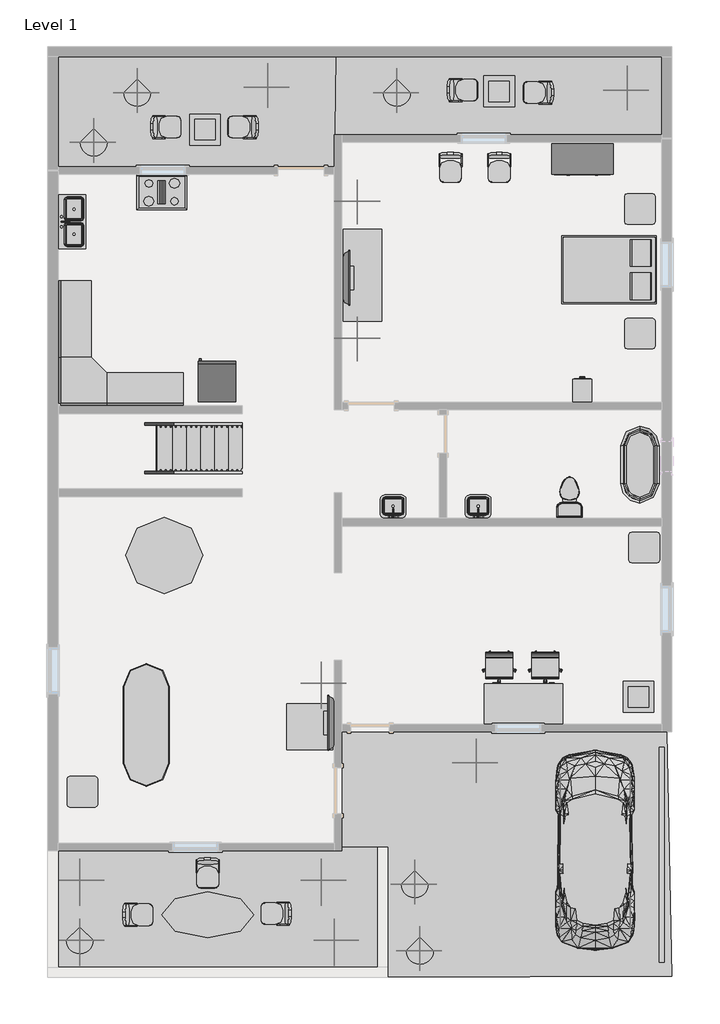
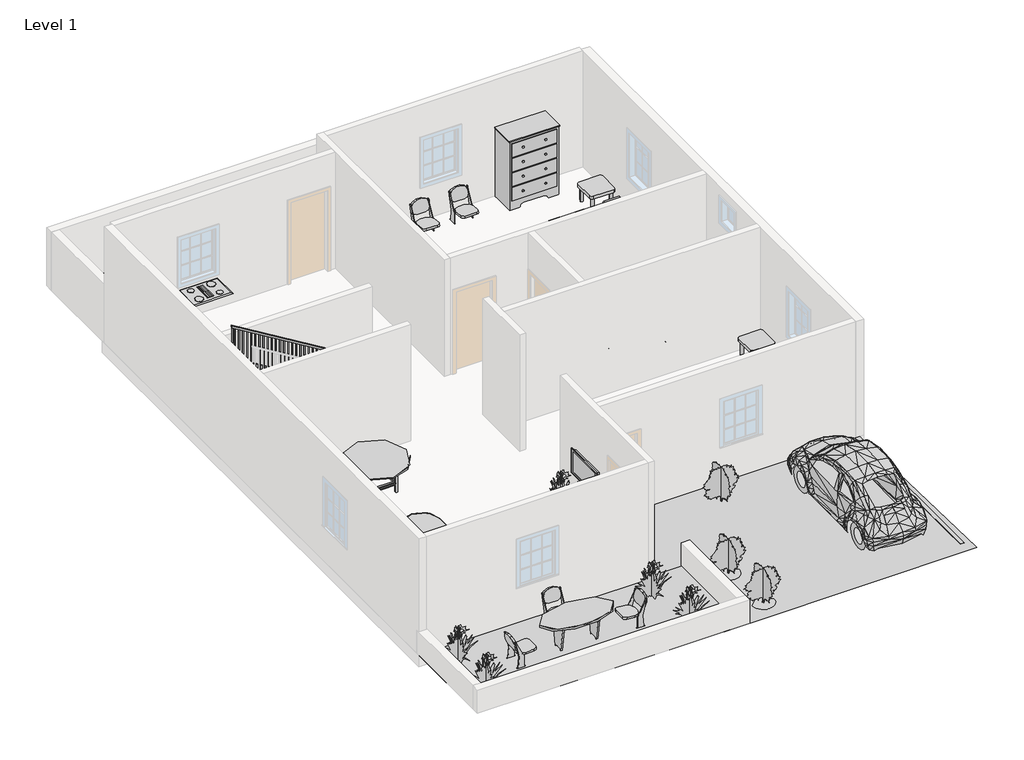
# One storey, part 2 of 2: 30 furniture elements, 15 geographic elements, 8 proxies, 6 flow terminals, 2 members, 1 railing, 1 stair flight.
"""IFC4 building model written with IfcOpenShell, lengths in millimetres."""

from ifc_helpers import new_model, si_unit, frame, origin, place, context, project, spatial, polyline, outline, extrude, triangles, transform, mapped, element, save
from components import proxy_bb1e6e30, parking_space_9_x_18_90_deg_fdd9e8f5, rpc_beetle_rpc_beetle_3ce7ba48, proxy_a13a33b2, flow_terminal_2b63360b, flow_terminal_a53be723, flow_terminal_62a433f7, toilet_domestic_3d_toilet_domestic_3d_f7549cf7, toilet_domestic_3d_toilet_domestic_3d_183bbd19, flow_terminal_b374fae2, furniture_1070mm_7a3aaa4f, furniture_c8abb964, furniture_552c1472, chair_task_chair_task_b7f3823b, furniture_013ab306, furniture_9fa109b2, m_table_rectangular_0915_x_0915mm_8578315f, furniture_3d1d9cbc, furniture_b5c51a22, furniture_e05f6f82, furniture_bbcc68ce, furniture_027a2ad9, furniture_5d68651d, furniture_a5b052b6, furniture_45e3acac, rpc_plant_tropical_55f6ff97, rpc_plant_tropical_agave_1_5_93a2a214, rpc_plant_tropical_jungle_flame_3_9c4808c2, stair_flight_159ea243

model = new_model("IFC4")

# Units and contexts
model_context = context("Model", 3, world=origin())
ifc_project = project(units=[si_unit("LENGTHUNIT", "METRE", prefix="MILLI")], contexts=[model_context])

# Site, building, storey
site = spatial("IfcSite", under=ifc_project)
building = spatial("IfcBuilding", under=site)
storey = spatial("IfcBuildingStorey", under=building, Name="Level 1", Elevation=0.0)

# Proxies
placement = place(None, origin())
element("IfcBuildingElementProxy", 1, Name="Building Element Proxy", at=placement, inside=storey, context=model_context, shape_type="Tessellation", body=[
    triangles([(-6254.9251831, -3080.6256248, 0.0), (-6254.9251831, -5671.4259155, 0.0), (501.4745868, -5671.4259155, 0.0), (501.4745868, -3080.6256248, 0.0), (-412.9254132, -3156.8256248, 0.0)], [[1, 2, 5], [5, 3, 4], [3, 5, 2], [5, 4, 1]], closed=False),
])
element("IfcBuildingElementProxy", 2, Name="Building Element Proxy", at=placement, inside=storey, context=model_context, shape_type="Tessellation", body=[
    triangles([(-412.9254132, -794.6256975, 0.0), (-412.9254132, -3156.8256248, 0.0), (6040.245845, -794.6256975, 0.0), (6140.2746231, -5646.0257217, 0.0), (501.4745868, -5671.4259155, 0.0), (-235.1254193, -693.0257217, 0.0), (526.8745989, -693.0257217, 0.0), (-514.5254253, -1505.8256733, 0.0), (-514.5254253, -2420.2256733, 0.0)], [[7, 8, 9], [6, 1, 8], [9, 2, 7], [5, 4, 3], [7, 6, 8], [2, 3, 7], [2, 5, 3]], closed=False),
])
element("IfcBuildingElementProxy", 3, Name="Building Element Proxy", at=placement, inside=storey, context=model_context, shape_type="Tessellation", body=[
    triangles([(-6051.7253769, 12616.5740845, 0.0), (-6051.7253769, 10432.1736969, 0.0), (-565.3254132, 10432.1736969, 0.0), (-533.6047113, 12616.5740845, 0.0)], [[1, 2, 3], [3, 4, 1]], closed=False),
])
element("IfcBuildingElementProxy", 4, Name="Building Element Proxy", at=placement, inside=storey, context=model_context, shape_type="Tessellation", body=[
    triangles([(-565.3254132, 11067.174472, 0.0), (-561.2836905, 12616.5740845, 0.0), (5937.0748169, 11067.174472, 0.0), (5937.0748169, 12616.5740845, 0.0)], [[2, 1, 3], [3, 4, 2]], closed=False),
])
proxy_shape = proxy_bb1e6e30(model_context)
element("IfcBuildingElementProxy", 5, Name="Cook Top-4 Unit : 36\" x 20\"", ObjectType="Cook Top-4 Unit : 36\" x 20\"", at=placement, inside=storey, context=model_context, shape_type="MappedRepresentation", body=[
    mapped(proxy_shape, transform((-3994.3254147, 9924.1742707, 0.0), x_axis=(1.0, 0.0, 0.0), y_axis=(0.0, 1.0, 0.0), z_axis=(0.0, 0.0, 1.0))),
])
parking_space_9_x_18_90_deg_shape = parking_space_9_x_18_90_deg_fdd9e8f5(model_context)
element("IfcBuildingElementProxy", 6, Name="Parking Space : 9' x 18' - 90 deg", ObjectType="Parking Space : 9' x 18' - 90 deg", at=placement, inside=storey, context=model_context, shape_type="MappedRepresentation", body=[
    mapped(parking_space_9_x_18_90_deg_shape, transform((5937.0745853, -5366.6257293, 0.0), x_axis=(-1.0000000000000004, 0.0, 0.0), y_axis=(0.0, -1.0000000000000004, 0.0), z_axis=(0.0, 0.0, 1.0))),
])
rpc_beetle_rpc_beetle_shape = rpc_beetle_rpc_beetle_3ce7ba48(model_context)
element("IfcBuildingElementProxy", 7, Name="RPC Beetle : RPC Beetle", ObjectType="RPC Beetle : RPC Beetle", at=placement, inside=storey, context=model_context, shape_type="MappedRepresentation", body=[
    mapped(rpc_beetle_rpc_beetle_shape, transform((4616.2745853, -4376.0257293, 0.0), x_axis=(1.0, 0.0, 0.0), y_axis=(0.0, 1.0, 0.0), z_axis=(0.0, 0.0, 1.0))),
])
proxy_2_shape = proxy_a13a33b2(model_context)
element("IfcBuildingElementProxy", 8, Name="Refrigerator : 30\" x 32\" RH", ObjectType="Refrigerator : 30\" x 32\" RH", at=placement, inside=storey, context=model_context, shape_type="MappedRepresentation", body=[
    mapped(proxy_2_shape, transform((-2894.1879147, 6151.0752993, 0.0), x_axis=(-1.0000000000000004, 0.0, 0.0), y_axis=(0.0, -1.0000000000000004, 0.0), z_axis=(0.0, 0.0, 1.0))),
])

# Flow terminals
flow_terminal_shape = flow_terminal_2b63360b(model_context)
element("IfcFlowTerminal", 9, ObjectType="Floor Drain - Rectangular : 5\"x5\" Strainer - 2\" Drain", at=placement, inside=storey, context=model_context, shape_type="MappedRepresentation", body=[
    mapped(flow_terminal_shape, transform((4819.4745853, 5225.1742707, 0.0), x_axis=(1.0, 0.0, 0.0), y_axis=(0.0, 1.0, 0.0), z_axis=(0.0, 0.0, 1.0))),
])
flow_terminal_2_shape = flow_terminal_a53be723(model_context)
element("IfcFlowTerminal", 10, ObjectType="Sink Kitchen-Double : 42\" x 21\"", at=placement, inside=storey, context=model_context, shape_type="MappedRepresentation", body=[
    mapped(flow_terminal_2_shape, transform((-5769.9800135, 9324.2850302, 0.0), x_axis=(0.0, 1.0000000000000002, 0.0), y_axis=(-1.0000000000000002, 0.0, 0.0), z_axis=(0.0, 0.0, 1.0))),
])
flow_terminal_3_shape = flow_terminal_62a433f7(model_context)
element("IfcFlowTerminal", 11, ObjectType="Sink Vanity-Square : 20\" x 18\"", at=placement, inside=storey, context=model_context, shape_type="MappedRepresentation", body=[
    mapped(flow_terminal_3_shape, transform((2307.8638259, 3640.0196719, 0.0), x_axis=(-1.0000000000000002, 0.0, 0.0), y_axis=(0.0, -1.0000000000000002, 0.0), z_axis=(0.0, 0.0, 1.0))),
])
element("IfcFlowTerminal", 12, ObjectType="Sink Vanity-Square : 20\" x 18\"", at=placement, inside=storey, context=model_context, shape_type="MappedRepresentation", body=[
    mapped(flow_terminal_3_shape, transform((618.7638259, 3640.0196719, 0.0), x_axis=(-1.0, 0.0, 0.0), y_axis=(0.0, -1.0, 0.0), z_axis=(0.0, 0.0, 1.0))),
])
toilet_domestic_3d_toilet_domestic_3d_shape = toilet_domestic_3d_toilet_domestic_3d_f7549cf7(model_context)
toilet_domestic_3d_toilet_domestic_3d_2_shape = toilet_domestic_3d_toilet_domestic_3d_183bbd19(model_context)
element("IfcFlowTerminal", 13, ObjectType="Toilet-Domestic-3D : Toilet-Domestic-3D", at=placement, inside=storey, context=model_context, shape_type="MappedRepresentation", body=[
    mapped(toilet_domestic_3d_toilet_domestic_3d_shape, transform((4108.2745853, 3967.2702981, 0.0), x_axis=(-0.9999999999999998, 0.0, 0.0), y_axis=(0.0, -0.9999999999999998, 0.0), z_axis=(0.0, 0.0, 1.0))),
    mapped(toilet_domestic_3d_toilet_domestic_3d_2_shape, transform((4108.2745853, 3967.2702981, 0.0), x_axis=(-0.9999999999999998, 0.0, 0.0), y_axis=(0.0, -0.9999999999999998, 0.0), z_axis=(0.0, 0.0, 1.0))),
])
flow_terminal_4_shape = flow_terminal_b374fae2(model_context)
element("IfcFlowTerminal", 14, ObjectType="Tub-Free Standing-3D : 30\" x 60\"", at=placement, inside=storey, context=model_context, shape_type="MappedRepresentation", body=[
    mapped(flow_terminal_4_shape, transform((5505.2745853, 4513.9742707, 0.0), x_axis=(1.0, 0.0, 0.0), y_axis=(0.0, 1.0, 0.0), z_axis=(0.0, 0.0, 1.0))),
])

# Furniture
furniture_1070mm_shape = furniture_1070mm_7a3aaa4f(model_context)
element("IfcFurniture", 15, ObjectType="1070mm", at=placement, inside=storey, context=model_context, shape_type="MappedRepresentation", body=[
    mapped(furniture_1070mm_shape, transform((-623.8640383, -620.7702434, 914.4), x_axis=(0.0, -1.0000000000000004, 0.0), y_axis=(1.0000000000000004, 0.0, 0.0), z_axis=(0.0, 0.0, 1.0))),
])
furniture_shape = furniture_c8abb964(model_context)
element("IfcFurniture", 16, ObjectType="Bed-Box : Double 53\" x 74\"", at=placement, inside=storey, context=model_context, shape_type="MappedRepresentation", body=[
    mapped(furniture_shape, transform((5130.1040935, 8726.6267298, 0.0), x_axis=(0.0, -1.0000000000000004, 0.0), y_axis=(1.0000000000000004, 0.0, 0.0), z_axis=(0.0, 0.0, 1.0))),
])
furniture_2_shape = furniture_552c1472(model_context)
element("IfcFurniture", 17, ObjectType="Cabinet-File 3 Drawer : 15\" x 18\"", at=placement, inside=storey, context=model_context, shape_type="MappedRepresentation", body=[
    mapped(furniture_2_shape, transform((4234.3781383, 5845.0399706, 0.0), x_axis=(-1.0, 0.0, 0.0), y_axis=(0.0, -1.0, 0.0), z_axis=(0.0, 0.0, 1.0))),
])
chair_task_chair_task_shape = chair_task_chair_task_b7f3823b(model_context)
element("IfcFurniture", 18, ObjectType="Chair-Task : Chair-Task", at=placement, inside=storey, context=model_context, shape_type="MappedRepresentation", body=[
    mapped(chair_task_chair_task_shape, transform((2852.265405, 545.1201724, 0.0), x_axis=(-1.000000000000001, 0.0, 0.0), y_axis=(0.0, -1.000000000000001, 0.0), z_axis=(0.0, 0.0, 1.0))),
])
element("IfcFurniture", 19, ObjectType="Chair-Task : Chair-Task", at=placement, inside=storey, context=model_context, shape_type="MappedRepresentation", body=[
    mapped(chair_task_chair_task_shape, transform((3766.665405, 545.1201724, 0.0), x_axis=(-1.0000000000000004, 0.0, 0.0), y_axis=(0.0, -1.0000000000000004, 0.0), z_axis=(0.0, 0.0, 1.0))),
])
furniture_3_shape = furniture_013ab306(model_context)
element("IfcFurniture", 20, ObjectType="Desk : 60\" x 30\" Student", at=placement, inside=storey, context=model_context, shape_type="MappedRepresentation", body=[
    mapped(furniture_3_shape, transform((3955.8745853, 145.1742707, 0.0), x_axis=(-1.0000000000000009, 0.0, 0.0), y_axis=(0.0, -1.0000000000000009, 0.0), z_axis=(0.0, 0.0, 1.0))),
])
furniture_4_shape = furniture_9fa109b2(model_context)
element("IfcFurniture", 21, ObjectType="Dresser : 48\" x 72\" x 24\"", at=placement, inside=storey, context=model_context, shape_type="MappedRepresentation", body=[
    mapped(furniture_4_shape, transform((4631.4678452, 10947.7372248, 0.0), x_axis=(1.0, 0.0, 0.0), y_axis=(0.0, 1.0, 0.0), z_axis=(0.0, 0.0, 1.0))),
])
m_table_rectangular_0915_x_0915mm_shape = m_table_rectangular_0915_x_0915mm_8578315f(model_context)
element("IfcFurniture", 22, ObjectType="M_Table-Rectangular : 0915 x 0915mm", at=placement, inside=storey, context=model_context, shape_type="MappedRepresentation", body=[
    mapped(m_table_rectangular_0915_x_0915mm_shape, transform((-1047.9254147, -693.0257293, 0.0), x_axis=(1.0, 0.0, 0.0), y_axis=(0.0, 1.0, 0.0), z_axis=(0.0, 0.0, 1.0))),
])
furniture_5_shape = furniture_3d1d9cbc(model_context)
element("IfcFurniture", 23, ObjectType="Seating-Auditorium : 18\" x 24\" x 30\"", at=placement, inside=storey, context=model_context, shape_type="MappedRepresentation", body=[
    mapped(furniture_5_shape, transform((1906.8024542, 10622.0496806, 0.0), x_axis=(-1.0, 0.0, 0.0), y_axis=(0.0, -1.0, 0.0), z_axis=(0.0, 0.0, 1.0))),
])
element("IfcFurniture", 24, ObjectType="Seating-Auditorium : 18\" x 24\" x 30\"", at=placement, inside=storey, context=model_context, shape_type="MappedRepresentation", body=[
    mapped(furniture_5_shape, transform((2872.0024542, 10622.0496806, 0.0), x_axis=(-1.0, 0.0, 0.0), y_axis=(0.0, -1.0, 0.0), z_axis=(0.0, 0.0, 1.0))),
])
element("IfcFurniture", 25, ObjectType="Seating-Auditorium : 18\" x 24\" x 30\"", at=placement, inside=storey, context=model_context, shape_type="MappedRepresentation", body=[
    mapped(furniture_5_shape, transform((-1518.4500048, -4562.1535981, 0.0), x_axis=(0.0, 1.0000000000000002, 0.0), y_axis=(-1.0000000000000002, 0.0, 0.0), z_axis=(0.0, 0.0, 1.0))),
])
element("IfcFurniture", 26, ObjectType="Seating-Auditorium : 18\" x 24\" x 30\"", at=placement, inside=storey, context=model_context, shape_type="MappedRepresentation", body=[
    mapped(furniture_5_shape, transform((-2919.1975458, -3398.7503194, 0.0), x_axis=(-1.0000000000000004, 0.0, 0.0), y_axis=(0.0, -1.0000000000000004, 0.0), z_axis=(0.0, 0.0, 1.0))),
])
element("IfcFurniture", 27, ObjectType="Seating-Auditorium : 18\" x 24\" x 30\"", at=placement, inside=storey, context=model_context, shape_type="MappedRepresentation", body=[
    mapped(furniture_5_shape, transform((-4666.8008245, -4266.0978604, 0.0), x_axis=(0.0, -1.0000000000000002, 0.0), y_axis=(1.0000000000000002, 0.0, 0.0), z_axis=(0.0, 0.0, 1.0))),
])
element("IfcFurniture", 28, ObjectType="Seating-Auditorium : 18\" x 24\" x 30\"", at=placement, inside=storey, context=model_context, shape_type="MappedRepresentation", body=[
    mapped(furniture_5_shape, transform((-4108.0008245, 11380.3021396, 0.0), x_axis=(0.0, -1.0000000000000002, 0.0), y_axis=(1.0000000000000002, 0.0, 0.0), z_axis=(0.0, 0.0, 1.0))),
])
element("IfcFurniture", 29, ObjectType="Seating-Auditorium : 18\" x 24\" x 30\"", at=placement, inside=storey, context=model_context, shape_type="MappedRepresentation", body=[
    mapped(furniture_5_shape, transform((-2178.8500048, 11058.8464019, 0.0), x_axis=(0.0, 1.0000000000000004, 0.0), y_axis=(-1.0000000000000004, 0.0, 0.0), z_axis=(0.0, 0.0, 1.0))),
])
element("IfcFurniture", 30, ObjectType="Seating-Auditorium : 18\" x 24\" x 30\"", at=placement, inside=storey, context=model_context, shape_type="MappedRepresentation", body=[
    mapped(furniture_5_shape, transform((1784.7991755, 12116.9021396, 0.0), x_axis=(0.0, -1.0000000000000004, 0.0), y_axis=(1.0000000000000004, 0.0, 0.0), z_axis=(0.0, 0.0, 1.0))),
])
element("IfcFurniture", 31, ObjectType="Seating-Auditorium : 18\" x 24\" x 30\"", at=placement, inside=storey, context=model_context, shape_type="MappedRepresentation", body=[
    mapped(furniture_5_shape, transform((3688.5499952, 11744.6464019, 0.0), x_axis=(0.0, 1.0000000000000004, 0.0), y_axis=(-1.0000000000000004, 0.0, 0.0), z_axis=(0.0, 0.0, 1.0))),
])
element("IfcFurniture", 32, ObjectType="TV - Flat Screen : 42\"", at=placement, inside=storey, context=model_context, shape_type="MappedRepresentation", body=[
    mapped(furniture_1070mm_shape, transform((-327.590231, 8226.3187849, 1041.4), x_axis=(0.0, 1.0000000000000002, 0.0), y_axis=(-1.0000000000000002, 0.0, 0.0), z_axis=(0.0, 0.0, 1.0))),
])
furniture_6_shape = furniture_b5c51a22(model_context)
element("IfcFurniture", 33, ObjectType="Table-Coffee : 24\" x 24\" x 24\"", at=placement, inside=storey, context=model_context, shape_type="MappedRepresentation", body=[
    mapped(furniture_6_shape, transform((5461.6088187, -191.3368071, 0.0), x_axis=(1.0, 0.0, 0.0), y_axis=(0.0, 1.0, 0.0), z_axis=(0.0, 0.0, 1.0))),
])
element("IfcFurniture", 34, ObjectType="Table-Coffee : 24\" x 24\" x 24\"", at=placement, inside=storey, context=model_context, shape_type="MappedRepresentation", body=[
    mapped(furniture_6_shape, transform((-3148.9911813, 11073.5631929, 0.0), x_axis=(1.0, 0.0, 0.0), y_axis=(0.0, 1.0, 0.0), z_axis=(0.0, 0.0, 1.0))),
])
element("IfcFurniture", 35, ObjectType="Table-Coffee : 24\" x 24\" x 24\"", at=placement, inside=storey, context=model_context, shape_type="MappedRepresentation", body=[
    mapped(furniture_6_shape, transform((2693.0088187, 11835.5631929, 0.0), x_axis=(1.0, 0.0, 0.0), y_axis=(0.0, 1.0, 0.0), z_axis=(0.0, 0.0, 1.0))),
])
furniture_7_shape = furniture_e05f6f82(model_context)
element("IfcFurniture", 36, ObjectType="Table-Dining Oval : 36\" x 96\" Glass Top", at=placement, inside=storey, context=model_context, shape_type="MappedRepresentation", body=[
    mapped(furniture_7_shape, transform((-4657.2237753, -253.1060571, 0.0), x_axis=(0.0, 1.0000000000000002, 0.0), y_axis=(-1.0000000000000002, 0.0, 0.0), z_axis=(0.0, 0.0, 1.0))),
])
furniture_8_shape = furniture_bbcc68ce(model_context)
element("IfcFurniture", 37, ObjectType="Table-Dining Round w Chairs : 60\" Diameter", at=placement, inside=storey, context=model_context, shape_type="MappedRepresentation", body=[
    mapped(furniture_8_shape, transform((-4047.2073819, 2895.4529593, 0.0), x_axis=(1.0, 0.0, 0.0), y_axis=(0.0, 1.0, 0.0), z_axis=(0.0, 0.0, 1.0))),
])
furniture_9_shape = furniture_027a2ad9(model_context)
element("IfcFurniture", 38, ObjectType="Table-Ellipse : 72\" x 36\"", at=placement, inside=storey, context=model_context, shape_type="MappedRepresentation", body=[
    mapped(furniture_9_shape, transform((-3079.9254147, -4426.8257293, 0.0), x_axis=(1.0, 0.0, 0.0), y_axis=(0.0, 1.0, 0.0), z_axis=(0.0, 0.0, 1.0))),
])
furniture_10_shape = furniture_5d68651d(model_context)
element("IfcFurniture", 39, ObjectType="Table-End : 24\" x 24\"", at=placement, inside=storey, context=model_context, shape_type="MappedRepresentation", body=[
    mapped(furniture_10_shape, transform((5196.7409551, 6965.0742707, 0.0), x_axis=(1.0, 0.0, 0.0), y_axis=(0.0, 1.0, 0.0), z_axis=(0.0, 0.0, 1.0))),
])
element("IfcFurniture", 40, ObjectType="Table-End : 24\" x 24\"", at=placement, inside=storey, context=model_context, shape_type="MappedRepresentation", body=[
    mapped(furniture_10_shape, transform((5196.7409551, 9441.5742707, 0.0), x_axis=(1.0, 0.0, 0.0), y_axis=(0.0, 1.0, 0.0), z_axis=(0.0, 0.0, 1.0))),
])
element("IfcFurniture", 41, ObjectType="Table-End : 24\" x 24\"", at=placement, inside=storey, context=model_context, shape_type="MappedRepresentation", body=[
    mapped(furniture_10_shape, transform((-5877.6590449, -2134.4757293, 0.0), x_axis=(1.0, 0.0, 0.0), y_axis=(0.0, 1.0, 0.0), z_axis=(0.0, 0.0, 1.0))),
])
element("IfcFurniture", 42, ObjectType="Table-End : 24\" x 24\"", at=placement, inside=storey, context=model_context, shape_type="MappedRepresentation", body=[
    mapped(furniture_10_shape, transform((5285.6409551, 2716.9242707, 0.0), x_axis=(1.0, 0.0, 0.0), y_axis=(0.0, 1.0, 0.0), z_axis=(0.0, 0.0, 1.0))),
])
furniture_11_shape = furniture_a5b052b6(model_context)
element("IfcFurniture", 43, ObjectType="Table-Rectangular : 72\" x 30\"", at=placement, inside=storey, context=model_context, shape_type="MappedRepresentation", body=[
    mapped(furniture_11_shape, transform((-6.5254147, 8273.1742707, 0.0), x_axis=(0.0, 1.0000000000000002, 0.0), y_axis=(-1.0000000000000002, 0.0, 0.0), z_axis=(0.0, 0.0, 1.0))),
])
furniture_12_shape = furniture_45e3acac(model_context)
element("IfcFurniture", 44, ObjectType="Work Station Cubicle : 96\" x 96\"", at=placement, inside=storey, context=model_context, shape_type="MappedRepresentation", body=[
    mapped(furniture_12_shape, transform((-6546.7484223, 5814.106023, 0.0), x_axis=(0.0, 1.0000000000000002, 0.0), y_axis=(-1.0000000000000002, 0.0, 0.0), z_axis=(0.0, 0.0, 1.0))),
])

# Geographic elements
rpc_plant_tropical_shape = rpc_plant_tropical_55f6ff97(model_context)
element("IfcGeographicElement", 45, ObjectType="RPC Plant - Tropical", at=placement, inside=storey, context=model_context, shape_type="MappedRepresentation", body=[
    mapped(rpc_plant_tropical_shape, transform((-819.3254147, 170.5742707, 0.0), x_axis=(1.0, 0.0, 0.0), y_axis=(0.0, 1.0, 0.0), z_axis=(0.0, 0.0, 1.0))),
])
element("IfcGeographicElement", 46, ObjectType="RPC Plant - Tropical", at=placement, inside=storey, context=model_context, shape_type="MappedRepresentation", body=[
    mapped(rpc_plant_tropical_shape, transform((-5619.9254147, -3741.0257293, 0.0), x_axis=(1.0, 0.0, 0.0), y_axis=(0.0, 1.0, 0.0), z_axis=(0.0, 0.0, 1.0))),
])
element("IfcGeographicElement", 47, ObjectType="RPC Plant - Tropical", at=placement, inside=storey, context=model_context, shape_type="MappedRepresentation", body=[
    mapped(rpc_plant_tropical_shape, transform((-819.3254147, -3741.0257293, 0.0), x_axis=(1.0, 0.0, 0.0), y_axis=(0.0, 1.0, 0.0), z_axis=(0.0, 0.0, 1.0))),
])
element("IfcGeographicElement", 48, ObjectType="RPC Plant - Tropical", at=placement, inside=storey, context=model_context, shape_type="MappedRepresentation", body=[
    mapped(rpc_plant_tropical_shape, transform((-5619.9254147, -4934.8257293, 0.0), x_axis=(1.0, 0.0, 0.0), y_axis=(0.0, 1.0, 0.0), z_axis=(0.0, 0.0, 1.0))),
])
element("IfcGeographicElement", 49, ObjectType="RPC Plant - Tropical", at=placement, inside=storey, context=model_context, shape_type="MappedRepresentation", body=[
    mapped(rpc_plant_tropical_shape, transform((-565.3254147, -4934.8257293, 0.0), x_axis=(1.0, 0.0, 0.0), y_axis=(0.0, 1.0, 0.0), z_axis=(0.0, 0.0, 1.0))),
])
rpc_plant_tropical_agave_1_5_shape = rpc_plant_tropical_agave_1_5_93a2a214(model_context)
element("IfcGeographicElement", 50, ObjectType="RPC Plant - Tropical : Agave - 1.5'", at=placement, inside=storey, context=model_context, shape_type="MappedRepresentation", body=[
    mapped(rpc_plant_tropical_agave_1_5_shape, transform((-108.1254147, 9746.3742707, 0.0), x_axis=(1.0, 0.0, 0.0), y_axis=(0.0, 1.0, 0.0), z_axis=(0.0, 0.0, 1.0))),
])
element("IfcGeographicElement", 51, ObjectType="RPC Plant - Tropical : Agave - 1.5'", at=placement, inside=storey, context=model_context, shape_type="MappedRepresentation", body=[
    mapped(rpc_plant_tropical_agave_1_5_shape, transform((-108.1254147, 7028.5742707, 0.0), x_axis=(1.0, 0.0, 0.0), y_axis=(0.0, 1.0, 0.0), z_axis=(0.0, 0.0, 1.0))),
])
rpc_plant_tropical_jungle_flame_3_shape = rpc_plant_tropical_jungle_flame_3_9c4808c2(model_context)
element("IfcGeographicElement", 52, ObjectType="RPC Plant - Tropical : Jungle Flame - 3'", at=placement, inside=storey, context=model_context, shape_type="MappedRepresentation", body=[
    mapped(rpc_plant_tropical_jungle_flame_3_shape, transform((-5340.5254147, 10914.7742707, 0.0), x_axis=(1.0, 0.0, 0.0), y_axis=(0.0, 1.0, 0.0), z_axis=(0.0, 0.0, 1.0))),
])
element("IfcGeographicElement", 53, ObjectType="RPC Plant - Tropical : Jungle Flame - 3'", at=placement, inside=storey, context=model_context, shape_type="MappedRepresentation", body=[
    mapped(rpc_plant_tropical_jungle_flame_3_shape, transform((-4476.9254147, 11905.3742707, 0.0), x_axis=(1.0, 0.0, 0.0), y_axis=(0.0, 1.0, 0.0), z_axis=(0.0, 0.0, 1.0))),
])
element("IfcGeographicElement", 54, ObjectType="RPC Plant - Tropical : Jungle Flame - 3'", at=placement, inside=storey, context=model_context, shape_type="MappedRepresentation", body=[
    mapped(rpc_plant_tropical_jungle_flame_3_shape, transform((-1886.1254147, 12006.9742707, 0.0), x_axis=(1.0, 0.0, 0.0), y_axis=(0.0, 1.0, 0.0), z_axis=(0.0, 0.0, 1.0))),
])
element("IfcGeographicElement", 55, ObjectType="RPC Plant - Tropical : Jungle Flame - 3'", at=placement, inside=storey, context=model_context, shape_type="MappedRepresentation", body=[
    mapped(rpc_plant_tropical_jungle_flame_3_shape, transform((679.2745853, 11905.3742707, 0.0), x_axis=(1.0, 0.0, 0.0), y_axis=(0.0, 1.0, 0.0), z_axis=(0.0, 0.0, 1.0))),
])
element("IfcGeographicElement", 56, ObjectType="RPC Plant - Tropical : Jungle Flame - 3'", at=placement, inside=storey, context=model_context, shape_type="MappedRepresentation", body=[
    mapped(rpc_plant_tropical_jungle_flame_3_shape, transform((5251.2745853, 11956.1742707, 0.0), x_axis=(1.0, 0.0, 0.0), y_axis=(0.0, 1.0, 0.0), z_axis=(0.0, 0.0, 1.0))),
])
element("IfcGeographicElement", 57, ObjectType="RPC Plant - Tropical : Jungle Flame - 3'", at=placement, inside=storey, context=model_context, shape_type="MappedRepresentation", body=[
    mapped(rpc_plant_tropical_jungle_flame_3_shape, transform((1034.8745853, -3817.2257293, 0.0), x_axis=(1.0, 0.0, 0.0), y_axis=(0.0, 1.0, 0.0), z_axis=(0.0, 0.0, 1.0))),
])
element("IfcGeographicElement", 58, ObjectType="RPC Plant - Tropical : Jungle Flame - 3'", at=placement, inside=storey, context=model_context, shape_type="MappedRepresentation", body=[
    mapped(rpc_plant_tropical_jungle_flame_3_shape, transform((2254.0745853, -1404.2257293, 0.0), x_axis=(1.0, 0.0, 0.0), y_axis=(0.0, 1.0, 0.0), z_axis=(0.0, 0.0, 1.0))),
])
element("IfcGeographicElement", 59, ObjectType="RPC Plant - Tropical : Jungle Flame - 3'", at=placement, inside=storey, context=model_context, shape_type="MappedRepresentation", body=[
    mapped(rpc_plant_tropical_jungle_flame_3_shape, transform((1136.4745853, -5138.0257293, 0.0), x_axis=(1.0, 0.0, 0.0), y_axis=(0.0, 1.0, 0.0), z_axis=(0.0, 0.0, 1.0))),
])

# Members
element("IfcMember", 60, ObjectType="Stringer - 2\" Width", at=placement, inside=storey, context=model_context, shape_type="SweptSolid", body=[
    extrude(outline(polyline([(25.0390838, -2390.4214984), (381.4478453, -2390.4214984), (2582.7811786, -6022.6214984), (2226.3724171, -6022.6214984), (25.0390838, -2390.4214984)])), frame((0.0, 4331.6166905, 0.0), z_axis=(0.0, 1.0, 0.0), x_axis=(0.0, 0.0, 1.0)), (0.0, 0.0, 1.0), 50.8),
])
element("IfcMember", 61, ObjectType="Stringer - 2\" Width", at=placement, inside=storey, context=model_context, shape_type="SweptSolid", body=[
    extrude(outline(polyline([(25.0390838, -2390.4214984), (381.4478453, -2390.4214984), (2582.7811786, -6022.6214984), (2226.3724171, -6022.6214984), (25.0390838, -2390.4214984)])), frame((0.0, 5296.8166905, 0.0), z_axis=(0.0, 1.0, 0.0), x_axis=(0.0, 0.0, 1.0)), (0.0, 0.0, 1.0), 50.8),
])

# Railing
element("IfcRailing", 62, ObjectType="Handrail - Rectangular", at=placement, inside=storey, context=model_context, shape_type="SweptSolid", body=[
    extrude(outline(polyline([(1193.6652064, -2390.4214984), (1253.0666667, -2390.4214984), (3454.4, -6022.6214984), (3394.9985397, -6022.6214984), (1193.6652064, -2390.4214984)])), frame((0.0, 5246.0166905, 0.0), z_axis=(0.0, 1.0, 0.0), x_axis=(0.0, 0.0, 1.0)), (0.0, 0.0, 1.0), 50.8),
    extrude(outline(polyline([(3343.0439943, -5936.8964984), (3354.5894488, -5955.9464984), (2370.6666667, -5955.9464984), (2370.6666667, -5936.8964984), (3343.0439943, -5936.8964984)])), frame((0.0, 5261.8916905, 0.0), z_axis=(0.0, 1.0, 0.0), x_axis=(0.0, 0.0, 1.0)), (0.0, 0.0, 1.0), 19.05),
    extrude(outline(polyline([(3281.4682367, -5835.2964984), (3293.0136913, -5854.3464984), (2370.6666667, -5854.3464984), (2370.6666667, -5835.2964984), (3281.4682367, -5835.2964984)])), frame((0.0, 5261.8916905, 0.0), z_axis=(0.0, 1.0, 0.0), x_axis=(0.0, 0.0, 1.0)), (0.0, 0.0, 1.0), 19.05),
    extrude(outline(polyline([(3219.8924791, -5733.6964984), (3231.4379337, -5752.7464984), (2370.6666667, -5752.7464984), (2370.6666667, -5733.6964984), (3219.8924791, -5733.6964984)])), frame((0.0, 5261.8916905, 0.0), z_axis=(0.0, 1.0, 0.0), x_axis=(0.0, 0.0, 1.0)), (0.0, 0.0, 1.0), 19.05),
    extrude(outline(polyline([(3158.3167216, -5632.0964984), (3169.8621761, -5651.1464984), (2201.3333333, -5651.1464984), (2201.3333333, -5632.0964984), (3158.3167216, -5632.0964984)])), frame((0.0, 5261.8916905, 0.0), z_axis=(0.0, 1.0, 0.0), x_axis=(0.0, 0.0, 1.0)), (0.0, 0.0, 1.0), 19.05),
    extrude(outline(polyline([(3096.740964, -5530.4964984), (3108.2864185, -5549.5464984), (2201.3333333, -5549.5464984), (2201.3333333, -5530.4964984), (3096.740964, -5530.4964984)])), frame((0.0, 5261.8916905, 0.0), z_axis=(0.0, 1.0, 0.0), x_axis=(0.0, 0.0, 1.0)), (0.0, 0.0, 1.0), 19.05),
    extrude(outline(polyline([(3035.1652064, -5428.8964984), (3046.710661, -5447.9464984), (2032.0, -5447.9464984), (2032.0, -5428.8964984), (3035.1652064, -5428.8964984)])), frame((0.0, 5261.8916905, 0.0), z_axis=(0.0, 1.0, 0.0), x_axis=(0.0, 0.0, 1.0)), (0.0, 0.0, 1.0), 19.05),
    extrude(outline(polyline([(2973.5894488, -5327.2964984), (2985.1349034, -5346.3464984), (2032.0, -5346.3464984), (2032.0, -5327.2964984), (2973.5894488, -5327.2964984)])), frame((0.0, 5261.8916905, 0.0), z_axis=(0.0, 1.0, 0.0), x_axis=(0.0, 0.0, 1.0)), (0.0, 0.0, 1.0), 19.05),
    extrude(outline(polyline([(2912.0136913, -5225.6964984), (2923.5591458, -5244.7464984), (2032.0, -5244.7464984), (2032.0, -5225.6964984), (2912.0136913, -5225.6964984)])), frame((0.0, 5261.8916905, 0.0), z_axis=(0.0, 1.0, 0.0), x_axis=(0.0, 0.0, 1.0)), (0.0, 0.0, 1.0), 19.05),
    extrude(outline(polyline([(2850.4379337, -5124.0964984), (2861.9833882, -5143.1464984), (1862.6666667, -5143.1464984), (1862.6666667, -5124.0964984), (2850.4379337, -5124.0964984)])), frame((0.0, 5261.8916905, 0.0), z_axis=(0.0, 1.0, 0.0), x_axis=(0.0, 0.0, 1.0)), (0.0, 0.0, 1.0), 19.05),
    extrude(outline(polyline([(2788.8621761, -5022.4964984), (2800.4076307, -5041.5464984), (1862.6666667, -5041.5464984), (1862.6666667, -5022.4964984), (2788.8621761, -5022.4964984)])), frame((0.0, 5261.8916905, 0.0), z_axis=(0.0, 1.0, 0.0), x_axis=(0.0, 0.0, 1.0)), (0.0, 0.0, 1.0), 19.05),
    extrude(outline(polyline([(2727.2864185, -4920.8964984), (2738.8318731, -4939.9464984), (1862.6666667, -4939.9464984), (1862.6666667, -4920.8964984), (2727.2864185, -4920.8964984)])), frame((0.0, 5261.8916905, 0.0), z_axis=(0.0, 1.0, 0.0), x_axis=(0.0, 0.0, 1.0)), (0.0, 0.0, 1.0), 19.05),
    extrude(outline(polyline([(2665.710661, -4819.2964984), (2677.2561155, -4838.3464984), (1693.3333333, -4838.3464984), (1693.3333333, -4819.2964984), (2665.710661, -4819.2964984)])), frame((0.0, 5261.8916905, 0.0), z_axis=(0.0, 1.0, 0.0), x_axis=(0.0, 0.0, 1.0)), (0.0, 0.0, 1.0), 19.05),
    extrude(outline(polyline([(2604.1349034, -4717.6964984), (2615.6803579, -4736.7464984), (1693.3333333, -4736.7464984), (1693.3333333, -4717.6964984), (2604.1349034, -4717.6964984)])), frame((0.0, 5261.8916905, 0.0), z_axis=(0.0, 1.0, 0.0), x_axis=(0.0, 0.0, 1.0)), (0.0, 0.0, 1.0), 19.05),
    extrude(outline(polyline([(2542.5591458, -4616.0964984), (2554.1046004, -4635.1464984), (1693.3333333, -4635.1464984), (1693.3333333, -4616.0964984), (2542.5591458, -4616.0964984)])), frame((0.0, 5261.8916905, 0.0), z_axis=(0.0, 1.0, 0.0), x_axis=(0.0, 0.0, 1.0)), (0.0, 0.0, 1.0), 19.05),
    extrude(outline(polyline([(2480.9833882, -4514.4964984), (2492.5288428, -4533.5464984), (1524.0, -4533.5464984), (1524.0, -4514.4964984), (2480.9833882, -4514.4964984)])), frame((0.0, 5261.8916905, 0.0), z_axis=(0.0, 1.0, 0.0), x_axis=(0.0, 0.0, 1.0)), (0.0, 0.0, 1.0), 19.05),
    extrude(outline(polyline([(2419.4076307, -4412.8964984), (2430.9530852, -4431.9464984), (1524.0, -4431.9464984), (1524.0, -4412.8964984), (2419.4076307, -4412.8964984)])), frame((0.0, 5261.8916905, 0.0), z_axis=(0.0, 1.0, 0.0), x_axis=(0.0, 0.0, 1.0)), (0.0, 0.0, 1.0), 19.05),
    extrude(outline(polyline([(2357.8318731, -4311.2964984), (2369.3773276, -4330.3464984), (1354.6666667, -4330.3464984), (1354.6666667, -4311.2964984), (2357.8318731, -4311.2964984)])), frame((0.0, 5261.8916905, 0.0), z_axis=(0.0, 1.0, 0.0), x_axis=(0.0, 0.0, 1.0)), (0.0, 0.0, 1.0), 19.05),
    extrude(outline(polyline([(2296.2561155, -4209.6964984), (2307.80157, -4228.7464984), (1354.6666667, -4228.7464984), (1354.6666667, -4209.6964984), (2296.2561155, -4209.6964984)])), frame((0.0, 5261.8916905, 0.0), z_axis=(0.0, 1.0, 0.0), x_axis=(0.0, 0.0, 1.0)), (0.0, 0.0, 1.0), 19.05),
    extrude(outline(polyline([(2234.6803579, -4108.0964984), (2246.2258125, -4127.1464984), (1354.6666667, -4127.1464984), (1354.6666667, -4108.0964984), (2234.6803579, -4108.0964984)])), frame((0.0, 5261.8916905, 0.0), z_axis=(0.0, 1.0, 0.0), x_axis=(0.0, 0.0, 1.0)), (0.0, 0.0, 1.0), 19.05),
    extrude(outline(polyline([(2173.1046004, -4006.4964984), (2184.6500549, -4025.5464984), (1185.3333333, -4025.5464984), (1185.3333333, -4006.4964984), (2173.1046004, -4006.4964984)])), frame((0.0, 5261.8916905, 0.0), z_axis=(0.0, 1.0, 0.0), x_axis=(0.0, 0.0, 1.0)), (0.0, 0.0, 1.0), 19.05),
    extrude(outline(polyline([(2111.5288428, -3904.8964984), (2123.0742973, -3923.9464984), (1185.3333333, -3923.9464984), (1185.3333333, -3904.8964984), (2111.5288428, -3904.8964984)])), frame((0.0, 5261.8916905, 0.0), z_axis=(0.0, 1.0, 0.0), x_axis=(0.0, 0.0, 1.0)), (0.0, 0.0, 1.0), 19.05),
    extrude(outline(polyline([(2049.9530852, -3803.2964984), (2061.4985397, -3822.3464984), (1185.3333333, -3822.3464984), (1185.3333333, -3803.2964984), (2049.9530852, -3803.2964984)])), frame((0.0, 5261.8916905, 0.0), z_axis=(0.0, 1.0, 0.0), x_axis=(0.0, 0.0, 1.0)), (0.0, 0.0, 1.0), 19.05),
    extrude(outline(polyline([(1988.3773276, -3701.6964984), (1999.9227822, -3720.7464984), (1016.0, -3720.7464984), (1016.0, -3701.6964984), (1988.3773276, -3701.6964984)])), frame((0.0, 5261.8916905, 0.0), z_axis=(0.0, 1.0, 0.0), x_axis=(0.0, 0.0, 1.0)), (0.0, 0.0, 1.0), 19.05),
    extrude(outline(polyline([(1926.80157, -3600.0964984), (1938.3470246, -3619.1464984), (1016.0, -3619.1464984), (1016.0, -3600.0964984), (1926.80157, -3600.0964984)])), frame((0.0, 5261.8916905, 0.0), z_axis=(0.0, 1.0, 0.0), x_axis=(0.0, 0.0, 1.0)), (0.0, 0.0, 1.0), 19.05),
    extrude(outline(polyline([(1865.2258125, -3498.4964984), (1876.771267, -3517.5464984), (1016.0, -3517.5464984), (1016.0, -3498.4964984), (1865.2258125, -3498.4964984)])), frame((0.0, 5261.8916905, 0.0), z_axis=(0.0, 1.0, 0.0), x_axis=(0.0, 0.0, 1.0)), (0.0, 0.0, 1.0), 19.05),
    extrude(outline(polyline([(1803.6500549, -3396.8964984), (1815.1955094, -3415.9464984), (846.6666667, -3415.9464984), (846.6666667, -3396.8964984), (1803.6500549, -3396.8964984)])), frame((0.0, 5261.8916905, 0.0), z_axis=(0.0, 1.0, 0.0), x_axis=(0.0, 0.0, 1.0)), (0.0, 0.0, 1.0), 19.05),
    extrude(outline(polyline([(1742.0742973, -3295.2964984), (1753.6197519, -3314.3464984), (846.6666667, -3314.3464984), (846.6666667, -3295.2964984), (1742.0742973, -3295.2964984)])), frame((0.0, 5261.8916905, 0.0), z_axis=(0.0, 1.0, 0.0), x_axis=(0.0, 0.0, 1.0)), (0.0, 0.0, 1.0), 19.05),
    extrude(outline(polyline([(1680.4985397, -3193.6964984), (1692.0439943, -3212.7464984), (677.3333333, -3212.7464984), (677.3333333, -3193.6964984), (1680.4985397, -3193.6964984)])), frame((0.0, 5261.8916905, 0.0), z_axis=(0.0, 1.0, 0.0), x_axis=(0.0, 0.0, 1.0)), (0.0, 0.0, 1.0), 19.05),
    extrude(outline(polyline([(1618.9227822, -3092.0964984), (1630.4682367, -3111.1464984), (677.3333333, -3111.1464984), (677.3333333, -3092.0964984), (1618.9227822, -3092.0964984)])), frame((0.0, 5261.8916905, 0.0), z_axis=(0.0, 1.0, 0.0), x_axis=(0.0, 0.0, 1.0)), (0.0, 0.0, 1.0), 19.05),
    extrude(outline(polyline([(1557.3470246, -2990.4964984), (1568.8924791, -3009.5464984), (677.3333333, -3009.5464984), (677.3333333, -2990.4964984), (1557.3470246, -2990.4964984)])), frame((0.0, 5261.8916905, 0.0), z_axis=(0.0, 1.0, 0.0), x_axis=(0.0, 0.0, 1.0)), (0.0, 0.0, 1.0), 19.05),
    extrude(outline(polyline([(1495.771267, -2888.8964984), (1507.3167216, -2907.9464984), (508.0, -2907.9464984), (508.0, -2888.8964984), (1495.771267, -2888.8964984)])), frame((0.0, 5261.8916905, 0.0), z_axis=(0.0, 1.0, 0.0), x_axis=(0.0, 0.0, 1.0)), (0.0, 0.0, 1.0), 19.05),
    extrude(outline(polyline([(1434.1955094, -2787.2964984), (1445.740964, -2806.3464984), (508.0, -2806.3464984), (508.0, -2787.2964984), (1434.1955094, -2787.2964984)])), frame((0.0, 5261.8916905, 0.0), z_axis=(0.0, 1.0, 0.0), x_axis=(0.0, 0.0, 1.0)), (0.0, 0.0, 1.0), 19.05),
    extrude(outline(polyline([(1372.6197519, -2685.6964984), (1384.1652064, -2704.7464984), (508.0, -2704.7464984), (508.0, -2685.6964984), (1372.6197519, -2685.6964984)])), frame((0.0, 5261.8916905, 0.0), z_axis=(0.0, 1.0, 0.0), x_axis=(0.0, 0.0, 1.0)), (0.0, 0.0, 1.0), 19.05),
    extrude(outline(polyline([(1311.0439943, -2584.0964984), (1322.5894488, -2603.1464984), (338.6666667, -2603.1464984), (338.6666667, -2584.0964984), (1311.0439943, -2584.0964984)])), frame((0.0, 5261.8916905, 0.0), z_axis=(0.0, 1.0, 0.0), x_axis=(0.0, 0.0, 1.0)), (0.0, 0.0, 1.0), 19.05),
    extrude(outline(polyline([(1249.4682367, -2482.4964984), (1261.0136913, -2501.5464984), (338.6666667, -2501.5464984), (338.6666667, -2482.4964984), (1249.4682367, -2482.4964984)])), frame((0.0, 5261.8916905, 0.0), z_axis=(0.0, 1.0, 0.0), x_axis=(0.0, 0.0, 1.0)), (0.0, 0.0, 1.0), 19.05),
    extrude(outline(polyline([(3383.4530852, -6003.5714984), (3394.9985397, -6022.6214984), (2370.6666667, -6022.6214984), (2370.6666667, -6003.5714984), (3383.4530852, -6003.5714984)])), frame((0.0, 5261.8916905, 0.0), z_axis=(0.0, 1.0, 0.0), x_axis=(0.0, 0.0, 1.0)), (0.0, 0.0, 1.0), 19.05),
    extrude(outline(polyline([(1193.6652064, -2390.4214984), (1205.210661, -2409.4714984), (338.6666667, -2409.4714984), (338.6666667, -2390.4214984), (1193.6652064, -2390.4214984)])), frame((0.0, 5261.8916905, 0.0), z_axis=(0.0, 1.0, 0.0), x_axis=(0.0, 0.0, 1.0)), (0.0, 0.0, 1.0), 19.05),
])

# Stair flight
stair_flight_shape = stair_flight_159ea243(model_context)
element("IfcStairFlight", 63, ObjectType="2\" Tread 1\" Nosing 1/4\" Riser", at=placement, inside=storey, context=model_context, shape_type="MappedRepresentation", body=[
    mapped(stair_flight_shape, transform((0.0, 0.0, 0.0), x_axis=(1.0, 0.0, 0.0), y_axis=(0.0, 1.0, 0.0), z_axis=(0.0, 0.0, 1.0))),
])

save(model, "model.ifc")

# Revit data of these elements
# Type "Cook Top-4 Unit : 36\" x 20\""
#   Assembly Code = "E1090400"
#   Depth = 2' - 0"
#   Width = 3' - 0"
#   Burner Material = Steel, Chrome Plated
#   Cooktop Material = Steel, Polished
#   Default Elevation = 0
# Type "Parking Space : 9' x 18' - 90 deg"
#   Angle = 90.00°
#   Parking Length = 18' - 0"
#   Parking Width = 9' - 0"
#   pl = 14' - 0"
#   pw = 9' - 0"
# Type "RPC Beetle : RPC Beetle"
#   built-in parameter 1005195 = "RPC-16-0U6E-L4EG-ENH1-J3KF-SVEL-0TX4-C0"
#   Height = 0
# Type "Refrigerator : 30\" x 32\" RH"
#   Label = "REF."
#   Assembly Code = "E1090400"
#   Depth = 2' - 7 3/4"
#   Handle = 2' - 3"
#   Height = 5' - 10"
#   Rear Clearance = 0' - 2"
#   Top Door Height = 1' - 8"
#   Width = 2' - 5 3/8"
#   Material = Steel, Paint Finish, Ivory, Glossy
#   Default Elevation = 0
# Type "Floor Drain - Rectangular : 5\"x5\" Strainer - 2\" Drain"
#   WFU = 2
#   Strainer Height = 0' - 3 1/4"
#   Half Strainer Length = 0' - 2 1/2"
#   Strainer Length = 0' - 5"
#   Radius 2 = 0' - 3.04167"
#   Radius 1 = 0' - 2.02083"
#   Radius 3 = 0' - 2 1/32"
#   Pipe Radius = 1"
#   Pipe Diameter = 2"
#   Height 2 = 0' - 0.725"
#   Height 1 = 0' - 1 13/16"
#   Body Radius = 0' - 4 1/16"
#   Body Height = 0' - 3 5/8"
#   Body Diameter = 0' - 8 1/8"
#   Drain Material = none
#   HWFU = 0
#   Default Elevation = 0
#   CWFU = 0
# Type "Sink Kitchen-Double : 42\" x 21\""
#   Assembly Code = "D2010410"
#   Counter Height = 3' - 0"
#   Depth = 1' - 9"
#   Width = 3' - 6"
#   Faucet Material = Steel, Polished
#   Sink Material = Steel, Polished
#   Default Elevation = 0
# Type "Sink Vanity-Square : 20\" x 18\""
#   Assembly Code = "D2010400"
#   Counter Height = 2' - 7"
#   Depth = 1' - 6"
#   Width = 1' - 8"
#   Basin Material = Porcelain, Linen
#   Faucet Material = Steel, Polished
#   Default Elevation = 0
# Type "Toilet-Domestic-3D : Toilet-Domestic-3D"
#   Assembly Code = "D2010110"
#   Toilet - Bowl/Basin Material = Porcelain, Linen
#   Toilet - Seat Material = Laminate, Linen, Matte
#   Default Elevation = 0
# Type "Tub-Free Standing-3D : 30\" x 60\""
#   Assembly Code = "D2010110"
#   Height = 1' - 6"
#   Length = 5' - 0"
#   Width = 2' - 6"
#   Tub Material = Porcelain, Ivory
#   Default Elevation = 0
# Type "1070mm"
#   SinAng = 0' - 0.0193"
#   L = 3' - 0.71517"
#   H = 1' - 8.65418"
#   Thickness = 0' - 4.33071"
#   Diagonal = 3' - 6.12598"
#   CosAng = 0' - 0.03431"
#   Stand [instance default] = yes
#   Default Elevation = 0
# Type "Bed-Box : Double 53\" x 74\""
#   Assembly Code = "E2020200"
#   Length = 6' - 2"
#   Width = 4' - 5"
#   Frame Material = Birch
#   Mattress Material = Linen, White
#   Default Elevation = 0
# Type "Cabinet-File 3 Drawer : 15\" x 18\""
#   Assembly Code = "E2020200"
#   Depth = 1' - 6"
#   Height = 3' - 5"
#   Width = 1' - 3"
#   Cabinet Material = Steel, Paint Finish, Ivory, Glossy
#   Handle Material = Steel, Chrome Plated
#   Default Elevation = 0
# Type "Chair-Task : Chair-Task"
#   Assembly Code = "E2020200"
#   Base Material = Plastic, Opaque Black
#   Caster Material = Plastic, Opaque Black
#   Seat/Back Material = Textile - Slate Blue
#   Default Elevation = 0
# Type "Desk : 60\" x 30\" Student"
#   Assembly Code = "E2020200"
#   Depth = 2' - 6"
#   Height = 2' - 6"
#   Leg Height = 0' - 6"
#   Width = 5' - 0"
#   Body Material = Laminate, Ivory, Matte
#   Handle/Leg Material = Steel, Chrome Plated
#   Top Material = Cherry
#   Default Elevation = 0
# Type "Dresser : 48\" x 72\" x 24\""
#   Assembly Code = "E2020200"
#   Depth = 2' - 0"
#   Height = 6' - 0"
#   Width = 4' - 0"
#   Dresser Material = Laminate - Ivory, Glossy
#   Drawer Material = Laminate, Ivory, Matte
#   Knob Material = Cherry
#   Default Elevation = 0
# Type "M_Table-Rectangular : 0915 x 0915mm"
#   Height = 2' - 6"
#   Length = 3' - 0.02362"
#   Width = 3' - 0.02362"
#   Base Material = Birch
#   Top Material = Birch
#   Default Elevation = 0
# Type "Seating-Auditorium : 18\" x 24\" x 30\""
#   Assembly Code = "E2020200"
#   Seat Material = Linen, Beige
#   Frame Material = Steel, Paint Finish, Dark Gray, Matte
#   Default Elevation = 0
# Type "TV - Flat Screen : 42\""
#   SinAng = 0' - 0.0193"
#   L = 3' - 0.71517"
#   H = 1' - 8.65418"
#   Thickness = 0' - 4.33071"
#   Diagonal = 3' - 6.12598"
#   CosAng = 0' - 0.03431"
#   Stand [instance default] = yes
#   Default Elevation = 0
# Type "Table-Coffee : 24\" x 24\" x 24\""
#   Assembly Code = "E2020200"
#   Height = 2' - 0"
#   Length = 2' - 0"
#   Width = 2' - 0"
#   Top Material = none
#   Frame Material = none
#   Default Elevation = 0
# Type "Table-Dining Oval : 36\" x 96\" Glass Top"
#   Assembly Code = "E2020200"
#   Length = 8' - 0"
#   Width = 3' - 0"
#   Base Material = Steel, Chrome Plated
#   Top Material = Glass - Clear, Grey
#   Default Elevation = 0
#   Description = (empty or 0)
# Type "Table-Dining Round w Chairs : 60\" Diameter"
#   Assembly Code = "E2020200"
#   Radius = 2' - 6"
#   Diameter = 5' - 0"
#   Height = 2' - 6"
#   Chairs = 6
#   Base Material = Pine
#   Top Material = Laminate, Linen, Matte
#   Default Elevation = 0
# Type "Table-Ellipse : 72\" x 36\""
#   Assembly Code = "E2020200"
#   Half Width = 1' - 6"
#   Half Length = 3' - 0"
#   Height = 2' - 6"
#   Length = 6' - 0"
#   Width = 3' - 0"
#   Base Material = Birch
#   Top Material = Laminate - Black
#   Default Elevation = 0
# Type "Table-End : 24\" x 24\""
#   Assembly Code = "E2020200"
#   Height = 1' - 6"
#   Length = 2' - 0"
#   Width = 2' - 0"
#   Base Material = Birch
#   Top Material = Laminate, Ivory, Matte
#   Default Elevation = 0
# Type "Table-Rectangular : 72\" x 30\""
#   Assembly Code = "E2020200"
#   Height = 2' - 6"
#   Length = 6' - 0"
#   Width = 2' - 6"
#   Base Material = Birch
#   Top Material = Birch
#   Default Elevation = 0
# Type "Work Station Cubicle : 96\" x 96\""
#   Assembly Code = "E2020"
#   Desktop Height = 2' - 6"
#   Desktop1 Width = 2' - 0"
#   Desktop2 Width = 2' - 0"
#   Panel Height = 5' - 6"
#   Panel1 Length = 5' - 0"
#   Panel2 Length = 5' - 0"
#   Cube Panel Material = Textile - Light Gray
#   Work Top Material = Laminate, Ivory, Matte
#   Default Elevation = 0
# Type "RPC Plant - Tropical"
#   built-in parameter 1005198 = "{2, 15},{39, RPC-16-FWM5-GM7X-C67P-4000-ST1L-LVER-AU},{1, 0},{1, 0},{2, 13},{1, 8},{5, Color},{1, 0},{1, 0},{3, 0.8},{3, 0.8},{3, 0.8},{1, 8},{7, BBoxMin},{1, 0},{1, 0},{1, 0},{1, 0},{1, 0},{1, 8},{7, BBoxMax},{1, 0},{1, 0},{1, 0},{1, 0},{1, 0},{2, 11},{9, RPCTypeId},{1, 0},{1, 0},{39, RPC-16-FWM5-GM7X-C67P-4000-ST1L-LVER-AU},{1, 6},{14, RPCPlantHeight},{1, 0},{1, 0},{1, 3},{2, 11},{7, keyword},{1, 0},{1, 0},{35, :RPCs:Shrubs [General]:Geometry:RPC},{2, 11},{8, category},{1, 0},{1, 0},{16, Shrubs [General]},{2, 11},{12, LocalizedUID},{1, 0},{1, 0},{10, Crane Lily},{2, 14},{6, Height},{1, 0},{1, 0},{1, 3},{1, 2},{16, Cast Reflections},{1, 0},{1, 0},{1, 0},{1, 2},{12, Cast Shadows},{1, 0},{1, 0},{1, 1},{1, 2},{9, Lock View},{1, 0},{1, 0},{1, 0},{1, 4},{5, ViewC},{1, 0},{1, 0},{1, 0},{21, assetlibrary_base.fbx},{1, 5},"
#   built-in parameter 1005195 = "RPC-16-FWM5-GM7X-C67P-4000-ST1L-LVER-AU"
#   Assembly Code = "G2050500"
#   Height = 3' - 0"
#   Default Elevation = 0
# Type "RPC Plant - Tropical : Agave - 1.5'"
#   built-in parameter 1005198 = "{2, 15},{39, RPC-16-G1GJ-63FX-7K5P-N000-ST1L-LVER-AU},{1, 0},{1, 0},{2, 13},{1, 8},{5, Color},{1, 0},{1, 0},{3, 0.8},{3, 0.8},{3, 0.8},{1, 8},{7, BBoxMin},{1, 0},{1, 0},{1, 0},{1, 0},{1, 0},{1, 8},{7, BBoxMax},{1, 0},{1, 0},{1, 0},{1, 0},{1, 0},{2, 11},{9, RPCTypeId},{1, 0},{1, 0},{39, RPC-16-G1GJ-63FX-7K5P-N000-ST1L-LVER-AU},{1, 6},{14, RPCPlantHeight},{1, 0},{1, 0},{3, 1.5},{2, 11},{7, keyword},{1, 0},{1, 0},{35, :RPCs:Plants [General]:Geometry:RPC},{2, 11},{8, category},{1, 0},{1, 0},{16, Plants [General]},{2, 11},{12, LocalizedUID},{1, 0},{1, 0},{5, Agave},{2, 14},{6, Height},{1, 0},{1, 0},{3, 1.5},{1, 2},{16, Cast Reflections},{1, 0},{1, 0},{1, 0},{1, 2},{12, Cast Shadows},{1, 0},{1, 0},{1, 1},{1, 2},{9, Lock View},{1, 0},{1, 0},{1, 0},{1, 4},{5, ViewC},{1, 0},{1, 0},{1, 0},{21, assetlibrary_base.fbx},{1, 5},"
#   built-in parameter 1005195 = "RPC-16-G1GJ-63FX-7K5P-N000-ST1L-LVER-AU"
#   Type Comments = "Agave"
#   Assembly Code = "G2050500"
#   Height = 1' - 6"
#   Default Elevation = 0
# Type "RPC Plant - Tropical : Jungle Flame - 3'"
#   built-in parameter 1005198 = "{2, 15},{39, RPC-16-FUVJ-JWG0-MWGK-8000-ST1L-LVER-AU},{1, 0},{1, 0},{2, 13},{1, 8},{5, Color},{1, 0},{1, 0},{3, 0.8},{3, 0.8},{3, 0.8},{1, 8},{7, BBoxMin},{1, 0},{1, 0},{1, 0},{1, 0},{1, 0},{1, 8},{7, BBoxMax},{1, 0},{1, 0},{1, 0},{1, 0},{1, 0},{2, 11},{9, RPCTypeId},{1, 0},{1, 0},{39, RPC-16-FUVJ-JWG0-MWGK-8000-ST1L-LVER-AU},{1, 6},{14, RPCPlantHeight},{1, 0},{1, 0},{1, 3},{2, 11},{7, keyword},{1, 0},{1, 0},{35, :RPCs:Shrubs [General]:Geometry:RPC},{2, 11},{8, category},{1, 0},{1, 0},{16, Shrubs [General]},{2, 11},{12, LocalizedUID},{1, 0},{1, 0},{12, Jungle Flame},{2, 14},{6, Height},{1, 0},{1, 0},{1, 3},{1, 2},{16, Cast Reflections},{1, 0},{1, 0},{1, 0},{1, 2},{12, Cast Shadows},{1, 0},{1, 0},{1, 1},{1, 2},{9, Lock View},{1, 0},{1, 0},{1, 0},{1, 4},{5, ViewC},{1, 0},{1, 0},{1, 0},{21, assetlibrary_base.fbx},{1, 5},"
#   built-in parameter 1005195 = "RPC-16-FUVJ-JWG0-MWGK-8000-ST1L-LVER-AU"
#   Type Comments = "Jungle Flame"
#   Assembly Code = "G2050500"
#   Height = 3' - 0"
#   Default Elevation = 0
# Type "Handrail - Rectangular"
#   Assembly Code = "C2010400"
#   built-in parameter 1008612 = 0.0416667 (stored number, unit not read)
#   built-in parameter 1008611 = 0.0416667 (stored number, unit not read)
#   built-in parameter 1008609 = 0.333333 (stored number, unit not read)
#   built-in parameter 1008604 = 0.166667 (stored number, unit not read)
#   built-in parameter 1008603 = 0.166667 (stored number, unit not read)
#   Railing Height = 3' - 0"
#   built-in parameter 1008630 = 2
#   built-in parameter 1008610 = 2
#   built-in parameter 1008618 = Baluster - Square : 3/4"
# Elements 1, 2, 3, 4 (IfcBuildingElementProxy)
#   Material = none
#   Phase Created = New Construction
# Element 5 (IfcBuildingElementProxy, "Cook Top-4 Unit : 36\" x 20\"")
#   Phase Created = New Construction
#   Materials on its faces: "Steel, Chrome Plated", "Steel, Polished"
# Element 6 (IfcBuildingElementProxy, "Parking Space : 9' x 18' - 90 deg")
#   Phase Created = New Construction
#   Materials on its faces: "Parking Stripe"
# Element 7 (IfcBuildingElementProxy, "RPC Beetle : RPC Beetle")
#   Phase Created = New Construction
# Element 8 (IfcBuildingElementProxy, "Refrigerator : 30\" x 32\" RH")
#   Phase Created = New Construction
#   Materials on its faces: "Steel, Paint Finish, Ivory, Glossy", "Steel, Chrome Plated"
# Element 9 (IfcFlowTerminal, "Floor Drain - Rectangular : 5\"x5\" Strainer - 2\" Drain")
#   Mark = "6"
#   Phase Created = New Construction
# Element 10 (IfcFlowTerminal, "Sink Kitchen-Double : 42\" x 21\"")
#   Mark = "1"
#   Phase Created = New Construction
#   Materials on its faces: "Steel, Polished"
# Element 11 (IfcFlowTerminal, "Sink Vanity-Square : 20\" x 18\"")
#   Mark = "4"
#   Phase Created = New Construction
#   Materials on its faces: "Porcelain, Linen", "Steel, Polished"
# Element 12 (IfcFlowTerminal, "Sink Vanity-Square : 20\" x 18\"")
#   Mark = "5"
#   Phase Created = New Construction
#   Materials on its faces: "Porcelain, Linen", "Steel, Polished"
# Element 13 (IfcFlowTerminal, "Toilet-Domestic-3D : Toilet-Domestic-3D")
#   Mark = "3"
#   Phase Created = New Construction
#   Materials on its faces: "Porcelain, Linen", "Laminate, Linen, Matte"
# Element 14 (IfcFlowTerminal, "Tub-Free Standing-3D : 30\" x 60\"")
#   Mark = "2"
#   Phase Created = New Construction
#   Materials on its faces: "Porcelain, Ivory"
# Element 15 (IfcFurniture, "1070mm")
#   Stand = yes
#   Phase Created = New Construction
#   Materials on its faces: "TV - Black", "TV - Glass", "TV - Screen"
# Element 16 (IfcFurniture, "Bed-Box : Double 53\" x 74\"")
#   Phase Created = New Construction
#   Materials on its faces: "Birch", "Linen, White"
# Element 17 (IfcFurniture, "Cabinet-File 3 Drawer : 15\" x 18\"")
#   Phase Created = New Construction
#   Materials on its faces: "Steel, Chrome Plated", "Steel, Paint Finish, Ivory, Glossy"
# Elements 18, 19 (IfcFurniture, "Chair-Task : Chair-Task")
#   Phase Created = New Construction
#   Materials on its faces: "Plastic, Opaque Black", "Textile - Slate Blue"
# Element 20 (IfcFurniture, "Desk : 60\" x 30\" Student")
#   Phase Created = New Construction
#   Materials on its faces: "Steel, Chrome Plated", "Laminate, Ivory, Matte", "Cherry"
# Element 21 (IfcFurniture, "Dresser : 48\" x 72\" x 24\"")
#   Phase Created = New Construction
#   Materials on its faces: "Laminate, Ivory, Matte", "Cherry", "Laminate - Ivory, Glossy"
# Element 22 (IfcFurniture, "M_Table-Rectangular : 0915 x 0915mm")
#   Phase Created = New Construction
#   Materials on its faces: "Birch"
# Elements 23, 24, 25, 26, 27, 28, 29, 30, 31 (IfcFurniture, "Seating-Auditorium : 18\" x 24\" x 30\"")
#   Phase Created = New Construction
#   Materials on its faces: "Steel, Paint Finish, Dark Gray, Matte", "Linen, Beige"
# Element 32 (IfcFurniture, "TV - Flat Screen : 42\"")
#   Stand = yes
#   Phase Created = New Construction
#   Materials on its faces: "TV - Black", "TV - Glass", "TV - Screen"
# Elements 33, 34, 35 (IfcFurniture, "Table-Coffee : 24\" x 24\" x 24\"")
#   Phase Created = New Construction
#   Materials on its faces: "Glass - Clear, Grey"
# Element 36 (IfcFurniture, "Table-Dining Oval : 36\" x 96\" Glass Top")
#   Phase Created = New Construction
#   Materials on its faces: "Steel, Chrome Plated", "Glass - Clear, Grey"
# Element 37 (IfcFurniture, "Table-Dining Round w Chairs : 60\" Diameter")
#   Phase Created = New Construction
#   Materials on its faces: "Pine", "Laminate, Linen, Matte"
# Element 38 (IfcFurniture, "Table-Ellipse : 72\" x 36\"")
#   Phase Created = New Construction
#   Materials on its faces: "Birch", "Laminate - Black"
# Elements 39, 40, 41, 42 (IfcFurniture, "Table-End : 24\" x 24\"")
#   Phase Created = New Construction
#   Materials on its faces: "Laminate, Ivory, Matte", "Birch"
# Element 43 (IfcFurniture, "Table-Rectangular : 72\" x 30\"")
#   Phase Created = New Construction
#   Materials on its faces: "Birch"
# Element 44 (IfcFurniture, "Work Station Cubicle : 96\" x 96\"")
#   Phase Created = New Construction
#   Materials on its faces: "Textile - Light Gray", "Laminate, Ivory, Matte"
# Elements 45, 46, 47, 48, 49 (IfcGeographicElement, "RPC Plant - Tropical")
#   Phase Created = New Construction
# Elements 50, 51 (IfcGeographicElement, "RPC Plant - Tropical : Agave - 1.5'")
#   Phase Created = New Construction
# Elements 52, 53, 54, 55, 56, 57, 58, 59 (IfcGeographicElement, "RPC Plant - Tropical : Jungle Flame - 3'")
#   Phase Created = New Construction
# Elements 60, 61 (IfcMember, "Stringer - 2\" Width")
#   Phase Created = New Construction
# Element 62 (IfcRailing, "Handrail - Rectangular")
#   Phase Created = New Construction
# Element 63 (IfcStairFlight, "2\" Tread 1\" Nosing 1/4\" Riser")
#   Phase Created = New Construction
# Materials
#   "Steel, Chrome Plated": class "Metal", colour RGB 17 17 17, transparency 0, Description = "Chromiuim plated steel", Cost = 0
#   "Steel, Polished": class "Metal", colour RGB 57 57 57, transparency 0, Description = "Polished steel", Cost = 0
#   "Steel, Paint Finish, Ivory, Glossy": class "Metal", colour RGB 247 247 239, transparency 0, Description = "Steel, paint finish, ivory, glossy", Cost = 0
#   "Porcelain, Linen": class "Ceramic", colour RGB 249 239 230, transparency 0, Description = "Porcelain, linen", Cost = 0
#   "Laminate, Linen, Matte": class "Plastic", colour RGB 249 239 230, transparency 0, Description = "Plastic Laminate - Linen, Matte", Cost = 0
#   "Porcelain, Ivory": class "Ceramic", colour RGB 247 247 239, transparency 0, Description = "Porcelain, ivory", Cost = 0
#   "Birch": class "Wood", colour RGB 224 178 126, transparency 0, Description = "Betula Alleghaniensis", Cost = 0
#   "Linen, White": class "Textile", colour RGB 247 247 239, transparency 0, Description = "Linen, white", Cost = 0
#   "Plastic, Opaque Black": class "Plastic", colour RGB 0 0 0, transparency 0.7, Description = "Plastic, generic, opaque black", Cost = 0
